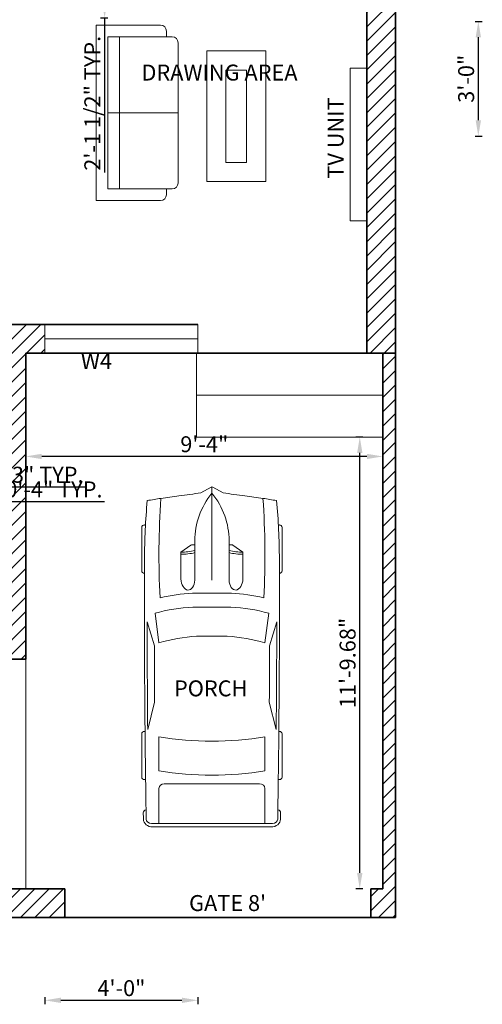
# Model space of a CAD drawing. Units: inches. Extents: x -196 to 219, y -474 to 80.
# Tile 3 of 4: x 73 to 219, y -456 to -148. Entities that reach past the tile are written whole.
import ezdxf

# ---------------------------------------------------------------- set-up
doc = ezdxf.new("R2010")
doc.units = ezdxf.units.IN
doc.header["$PDMODE"] = 35
doc.header["$PDSIZE"] = 5
for name, color, linetype, lineweight in [('A-ANNO-DIMS', 2, 'Continuous', 18), ('A-ANNO-TEXT', 7, 'Continuous', 18), ('A-AREA-IDEN', 7, 'Continuous', 25), ('A-FLOR-STRS', 3, 'Continuous', 18), ('A-GLAZ', 4, 'Continuous', 18), ('A-SITE-VEHI', 8, 'Continuous', 13), ('A-WALL', 7, 'Continuous', 35), ('A-WALL-PATT', 252, 'Continuous', 13), ('A-WALL-SITE', 7, 'Continuous', 35), ('furn', 28, 'Continuous', 18)]:
    doc.layers.add(name, color=color, linetype=linetype, lineweight=lineweight)
doc.styles.get("Standard").update_dxf_attribs({"font": 'arial.ttf'})
doc.dimstyles.new('ISO-25', dxfattribs={"dimtxt": 5, "dimasz": 5, "dimexe": 1.25, "dimexo": 0.625, "dimtad": 1, "dimlunit": 3, "dimtxsty": 'Standard', "dimcen": 2.5, "dimadec": 0, "dimazin": 0, "dimtfac": 1, "dimtmove": 0, "dimatfit": 3, "dimfxl": 1, "dimfxlon": 1, "dimarcsym": 0})

# ---------------------------------------------------------------- blocks, each defined once
blk = doc.blocks.new('sofa-6')
at = {"color": 0, "linetype": 'ByBlock'}
for p, q in [((1.35, 0.7), (0.15, 0.7)), ((0.75, 0.1), (0.75, 0.7)), ((0.1, 0.6), (0.05, 0.6)), ((0.1, 0.65), (0.1, 0.1)), ((1.4, 0.1), (1.4, 0.65)), ((1.45, 0.6), (1.4, 0.6)), ((0, 0.55), (0, 0)), ((1.5, 0), (1.5, 0.55)), ((0.1, 0.2), (1.4, 0.2)), ((0.1, 0.1), (1.4, 0.1)), ((0, 0), (1.5, 0))]:
    blk.add_line(p, q, dxfattribs=at)
for centre, start, end in [((0.15, 0.65), 90, 180), ((1.35, 0.65), 360, 90), ((0.05, 0.55), 90, 180), ((1.45, 0.55), 0, 90)]:
    blk.add_arc(centre, 0.05, start, end, dxfattribs=at)
blk = doc.blocks.new('*U24')
for p, q in [((46.55, 38.89), (22.35, 38.89)), ((136.7, 38.89), (160.9, 38.89)), ((21.1, 37.41), (21.1, 36.83)), ((47.8, 37.39), (47.8, 37.41)), ((87.99, 31.87), (74.76, 35.92)), ((134.31, 35.6), (119.29, 31.78)), ((135.45, 37.07), (135.45, 37.41)), ((162.15, 37.41), (162.15, 36.77)), ((186.47, -33.5), (186.47, 33.5)), ((188.4, -32.76), (188.4, 32.76)), ((70.03, 31.54), (86.41, 29.35)), ((138.42, 29.35), (157.25, 29.35)), ((186.47, 29.35), (167.01, 29.35)), ((164.52, 26.39), (164.52, -26.39)), ((32.27, 11.63), (36.13, 17.17)), ((36.13, 17.17), (50.94, 17.17)), ((32.12, 9.51), (32.12, 11.15)), ((3.27, 6.13), (0.1, 0.41)), ((29.77, 9.51), (51.68, 9.51)), ((58.92, -10.77), (58.92, 10.77)), ((66.55, -10.53), (66.55, 10.53)), ((82.74, 8.5), (82.74, -8.5)), ((186.47, -10.53), (186.47, 10.53)), ((0, 0), (51.68, 0)), ((0.1, -0.41), (3.27, -6.13)), ((29.77, -9.51), (51.68, -9.51)), ((32.12, -9.51), (32.12, -11.15)), ((32.27, -11.63), (36.13, -17.17)), ((36.13, -17.17), (50.94, -17.17)), ((86.41, -29.35), (70.03, -31.54)), ((87.99, -31.87), (74.76, -35.92)), ((134.31, -35.6), (119.29, -31.78)), ((157.25, -29.35), (138.42, -29.35)), ((167.01, -29.35), (186.47, -29.35)), ((21.1, -37.41), (21.1, -36.83)), ((47.8, -37.39), (47.8, -37.41)), ((135.45, -37.07), (135.45, -37.41)), ((162.15, -37.41), (162.15, -36.77)), ((46.55, -38.89), (22.35, -38.89)), ((136.7, -38.89), (160.9, -38.89))]:
    blk.add_line(p, q)
for centre, major_axis, ratio, start_param, end_param in [((22.35, 37.41), (0, -1.48), 0.842304, 3.141593, 4.712389), ((46.55, 37.41), (0, 1.48), 0.842304, -1.570796, 0), ((136.7, 37.41), (0, -1.48), 0.842304, 3.141593, 4.712389), ((160.9, 37.41), (0, 1.48), 0.842304, -1.570796, 0), ((266.03, -27.52), (0, 313.31), 0.842304, 1.367076, 1.39176), ((41.19, -490.86), (0, 528.23), 0.842304, 0.00281, 0.075598), ((64.48, -10555.62), (0, 10593.03), 0.842304, -0.013397, 0.002797), ((64.48, -10555.62), (0, -10591.55), 0.842304, 3.133765, 3.140441), ((180.63, 35.84), (0, 2.22), 0.842304, -0.013017, 1.249894), ((64.48, -10556.36), (0, 10595.31), 0.842304, -0.013397, -0.013017), ((183.98, 33.5), (0, -2.96), 0.842304, 1.570796, 3.128196), ((183.98, 32.76), (0, -5.25), 0.842304, 1.570796, 3.128196), ((259.18, -27.52), (0, -305.3), 0.842304, 4.528606, 4.561838), ((37.47, -593.96), (0, -623.33), 0.842304, 3.096046, 3.200911), ((134.4, 5.39), (0, -89.78), 0.842304, 4.449482, 4.652344), ((135.29, 5.39), (0, 81.77), 0.842304, 1.245306, 1.50788), ((149.6, 2.8), (0, -79.58), 0.842304, 4.372215, 4.640744), ((95.79, -3666.35), (0, -3698.24), 0.842304, 3.134049, 3.144098), ((17.08, 0), (0, 147.02), 0.842304, 4.511394, 4.913384), ((35.91, 0), (0, 147.02), 0.842304, 4.511394, 4.913384), ((167.01, 26.39), (0, 2.96), 0.842304, 0, 1.570796), ((-204.49, 52.4), (0, -250.96), 0.842304, 1.385369, 1.434372), ((13.04, 17.01), (0, 27.42), 0.842304, 4.435146, 4.718221), ((14.2, 17.01), (0, 27.42), 0.842304, 4.435146, 4.718221), ((50.79, 13.34), (6.34, -0.36), 0.603834, -1.395552, 1.581315), ((32.75, 11.15), (0, 0.74), 0.842304, 0.879714, 1.570796), ((29.77, -46.66), (0, 56.17), 0.842304, 0, 0.590319), ((0.62, 0), (0, -0.74), 0.842304, 4.131459, 5.293319), ((29.77, 46.66), (0, 56.17), 0.842304, 2.551274, 3.141593), ((-204.49, -52.4), (0, 250.96), 0.842304, -1.434372, -1.385369), ((13.04, -17.01), (0, -27.42), 0.842304, 1.564964, 1.848039), ((14.2, -17.01), (0, -27.42), 0.842304, 1.564964, 1.848039), ((134.4, -5.39), (0, -89.78), 0.842304, -1.510751, -1.307889), ((135.29, -5.39), (0, -81.77), 0.842304, -1.50788, -1.245306), ((149.6, -2.8), (0, -79.58), 0.842304, -1.499151, -1.230623), ((32.75, -11.15), (0, -0.74), 0.842304, 4.712389, 5.403472), ((259.18, 27.52), (0, 305.3), 0.842304, 1.721348, 1.754579), ((167.01, -26.39), (0, -2.96), 0.842304, 4.712389, 6.283185), ((266.03, 27.52), (0, 313.31), 0.842304, 1.749832, 1.774517), ((37.47, 593.96), (0, -623.33), 0.842304, -0.059319, 0.045547), ((95.79, 3666.35), (0, -3698.24), 0.842304, -0.002505, 0.007544), ((41.19, 490.86), (0, -528.23), 0.842304, -0.075598, -0.00281), ((22.35, -37.41), (0, 1.48), 0.842304, 1.570796, 3.141593), ((64.48, 10555.62), (0, 10593.03), 0.842304, 3.138796, 3.15499), ((46.55, -37.41), (0, -1.48), 0.842304, 0, 1.570796), ((64.48, 10555.62), (0, -10591.55), 0.842304, 0.001152, 0.007828), ((136.7, -37.41), (0, -1.48), 0.842304, -1.570796, 0), ((160.9, -37.41), (0, 1.48), 0.842304, 3.141593, 4.712389), ((180.63, -35.84), (0, -2.22), 0.842304, -1.249894, 0.013017), ((64.48, 10556.36), (0, 10595.31), 0.842304, 3.15461, 3.15499), ((183.98, -33.5), (0, 2.96), 0.842304, 3.15499, 4.712389), ((183.98, -32.76), (0, -5.25), 0.842304, 0.013397, 1.570796)]:
    blk.add_ellipse(centre, major_axis=major_axis, ratio=ratio, start_param=start_param, end_param=end_param)
at = {"extrusion": (0, 0, -1)}
blk.add_ellipse((50.79, -13.34), major_axis=(6.34, 0.36), ratio=0.603834, start_param=-1.395552, end_param=1.581315, dxfattribs=at)
blk = doc.blocks.new('*D27')
at = {"layer": 'A-ANNO-DIMS', "color": 0, "lineweight": -2, "transparency": 16777216}
for p, q in [((181.06, -278.42), (178.81, -278.42)), ((180.06, -415.09), (180.06, -283.42)), ((181.06, -420.09), (178.81, -420.09))]:
    blk.add_line(p, q, dxfattribs=at)
at = {"layer": 'A-ANNO-DIMS', "color": 0, "transparency": 16777216}
for points in [[(179.23, -283.42), (180.9, -283.42), (180.06, -278.42)], [(179.23, -415.09), (180.9, -415.09), (180.06, -420.09)]]:
    blk.add_solid(points, dxfattribs=at)
at = {"layer": 'Defpoints', "color": 0, "transparency": 16777216}
for p in [(180.06, -278.42), (187.3, -278.42), (187.3, -420.09)]:
    blk.add_point(p, dxfattribs=at)
at = {"layer": 'A-ANNO-DIMS', "color": 0, "transparency": 16777216, "insert": (176.89, -349.26), "char_height": 5, "attachment_point": 5, "rotation": 90}
blk.add_mtext('11\'-9.68"', dxfattribs=at)
blk = doc.blocks.new('*D28')
at = {"layer": 'A-ANNO-DIMS', "color": 0, "lineweight": -2, "transparency": 16777216}
for p, q in [((75.3, -284.51), (75.3, -283.26)), ((187.3, -283.51), (187.3, -285.76)), ((182.3, -284.51), (80.3, -284.51))]:
    blk.add_line(p, q, dxfattribs=at)
at = {"layer": 'A-ANNO-DIMS', "color": 0, "transparency": 16777216}
for points in [[(80.3, -283.68), (80.3, -285.34), (75.3, -284.51)], [(182.3, -283.68), (182.3, -285.34), (187.3, -284.51)]]:
    blk.add_solid(points, dxfattribs=at)
at = {"layer": 'Defpoints', "color": 0, "transparency": 16777216}
for p in [(187.3, -278.42), (75.3, -284.51), (75.3, -284.51)]:
    blk.add_point(p, dxfattribs=at)
at = {"layer": 'A-ANNO-DIMS', "color": 0, "transparency": 16777216, "insert": (131.3, -281.33), "char_height": 5, "attachment_point": 5}
blk.add_mtext('9\'-4"', dxfattribs=at)
blk = doc.blocks.new('*D45')
at = {"layer": 'A-ANNO-DIMS', "color": 0, "lineweight": -2, "transparency": 16777216}
for p, q in [((101.03, -121.37), (98.78, -121.37)), ((100.03, -126.37), (100.03, -142.04)), ((101.03, -147.04), (98.78, -147.04)), ((100.03, -147.04), (100.03, -195.5))]:
    blk.add_line(p, q, dxfattribs=at)
at = {"layer": 'A-ANNO-DIMS', "color": 0, "transparency": 16777216}
for points in [[(99.19, -126.37), (100.86, -126.37), (100.03, -121.37)], [(99.19, -142.04), (100.86, -142.04), (100.03, -147.04)]]:
    blk.add_solid(points, dxfattribs=at)
at = {"layer": 'Defpoints', "color": 0, "transparency": 16777216}
for p in [(108.28, -121.37), (100.03, -147.04), (108.28, -147.04)]:
    blk.add_point(p, dxfattribs=at)
at = {"layer": 'A-ANNO-DIMS', "color": 0, "transparency": 16777216, "insert": (96.82, -173.77), "char_height": 5, "attachment_point": 5, "rotation": 90}
blk.add_mtext('2\'-1 1/2" TYP.', dxfattribs=at)
blk = doc.blocks.new('*D49')
at = {"layer": 'A-ANNO-DIMS', "color": 0, "lineweight": -2, "transparency": 16777216}
for p, q in [((49.1, -298.67), (44.1, -298.67)), ((54.1, -298.67), (54.1, -299.92)), ((54.1, -298.67), (58.25, -298.67)), ((58.25, -298.67), (58.25, -299.92)), ((63.25, -298.67), (99.98, -298.67))]:
    blk.add_line(p, q, dxfattribs=at)
at = {"layer": 'A-ANNO-DIMS', "color": 0, "transparency": 16777216}
for points in [[(49.1, -297.83), (49.1, -299.5), (54.1, -298.67)], [(63.25, -297.83), (63.25, -299.5), (58.25, -298.67)]]:
    blk.add_solid(points, dxfattribs=at)
at = {"layer": 'Defpoints', "color": 0, "transparency": 16777216}
for p in [(54.1, -298.04), (58.25, -298.04), (58.25, -298.67)]:
    blk.add_point(p, dxfattribs=at)
at = {"layer": 'A-ANNO-DIMS', "color": 0, "transparency": 16777216, "insert": (84.11, -295.49), "char_height": 5, "attachment_point": 5}
blk.add_mtext('0\'-4" TYP.', dxfattribs=at)
blk = doc.blocks.new('*D51')
at = {"layer": 'A-ANNO-DIMS', "color": 0, "lineweight": -2, "transparency": 16777216}
for p, q in [((49.39, -294.07), (49.39, -292.82)), ((52.3, -294.07), (52.3, -292.82)), ((44.39, -294.07), (39.39, -294.07)), ((49.39, -294.07), (52.3, -294.07)), ((57.3, -294.07), (94.02, -294.07))]:
    blk.add_line(p, q, dxfattribs=at)
at = {"layer": 'A-ANNO-DIMS', "color": 0, "transparency": 16777216}
for points in [[(44.39, -293.23), (44.39, -294.9), (49.39, -294.07)], [(57.3, -293.23), (57.3, -294.9), (52.3, -294.07)]]:
    blk.add_solid(points, dxfattribs=at)
at = {"layer": 'Defpoints', "color": 0, "transparency": 16777216}
for p in [(49.39, -294.5), (52.3, -294.07), (52.3, -294.5)]:
    blk.add_point(p, dxfattribs=at)
at = {"layer": 'A-ANNO-DIMS', "color": 0, "transparency": 16777216, "insert": (78.16, -290.89), "char_height": 5, "attachment_point": 5}
blk.add_mtext('0\'-3" TYP.', dxfattribs=at)
blk = doc.blocks.new('*D56')
at = {"layer": 'A-ANNO-DIMS', "color": 0, "lineweight": -2, "transparency": 16777216}
for p, q in [((216.25, -148.09), (218.5, -148.09)), ((217.25, -153.09), (217.25, -179.09)), ((216.25, -184.09), (218.5, -184.09))]:
    blk.add_line(p, q, dxfattribs=at)
at = {"layer": 'A-ANNO-DIMS', "color": 0, "transparency": 16777216}
for points in [[(216.42, -153.09), (218.09, -153.09), (217.25, -148.09)], [(216.42, -179.09), (218.09, -179.09), (217.25, -184.09)]]:
    blk.add_solid(points, dxfattribs=at)
at = {"layer": 'Defpoints', "color": 0, "transparency": 16777216}
for p in [(-35.7, -148.09), (-35.7, -184.09), (217.25, -184.09)]:
    blk.add_point(p, dxfattribs=at)
at = {"layer": 'A-ANNO-DIMS', "color": 0, "transparency": 16777216, "insert": (214.07, -166.09), "char_height": 5, "attachment_point": 5, "rotation": 90}
blk.add_mtext('3\'-0"', dxfattribs=at)
blk = doc.blocks.new('*D59')
at = {"layer": 'A-ANNO-DIMS', "color": 0, "lineweight": -2, "transparency": 16777216}
for p, q in [((81.3, -454.04), (81.3, -456.29)), ((86.3, -455.04), (124.3, -455.04)), ((129.3, -454.04), (129.3, -456.29))]:
    blk.add_line(p, q, dxfattribs=at)
at = {"layer": 'A-ANNO-DIMS', "color": 0, "transparency": 16777216}
for points in [[(86.3, -454.21), (86.3, -455.88), (81.3, -455.04)], [(124.3, -454.21), (124.3, -455.88), (129.3, -455.04)]]:
    blk.add_solid(points, dxfattribs=at)
at = {"layer": 'Defpoints', "color": 0, "transparency": 16777216}
for p in [(81.3, -252.09), (129.3, -252.09), (129.3, -455.04)]:
    blk.add_point(p, dxfattribs=at)
at = {"layer": 'A-ANNO-DIMS', "color": 0, "transparency": 16777216, "insert": (105.3, -451.87), "char_height": 5, "attachment_point": 5}
blk.add_mtext('4\'-0"', dxfattribs=at)
blk = doc.blocks.new('*D60')
at = {"layer": 'A-ANNO-DIMS', "color": 0, "lineweight": -2, "transparency": 16777216}
for p, q in [((66.3, 72.61), (66.3, 74.86)), ((75.3, 72.61), (75.3, 74.86)), ((61.3, 73.61), (56.3, 73.61)), ((66.3, 73.61), (75.3, 73.61)), ((80.3, 73.61), (99.84, 73.61))]:
    blk.add_line(p, q, dxfattribs=at)
at = {"layer": 'A-ANNO-DIMS', "color": 0, "transparency": 16777216}
for points in [[(61.3, 74.45), (61.3, 72.78), (66.3, 73.61)], [(80.3, 74.45), (80.3, 72.78), (75.3, 73.61)]]:
    blk.add_solid(points, dxfattribs=at)
at = {"layer": 'Defpoints', "color": 0, "transparency": 16777216}
for p in [(75.3, 73.61), (66.3, -339.09), (75.3, -348.09)]:
    blk.add_point(p, dxfattribs=at)
at = {"layer": 'A-ANNO-DIMS', "color": 0, "transparency": 16777216, "insert": (92.57, 76.79), "char_height": 5, "attachment_point": 5}
blk.add_mtext('0\'-9"', dxfattribs=at)

msp = doc.modelspace()

# ---------------------------------------------------------------- hatches: boundary and pattern name
at = {"layer": 'A-WALL-PATT'}
h = msp.add_hatch(dxfattribs=at)
h.set_pattern_fill('ANSI31', color=256)
h.set_pattern_definition([(45, (-560.5042, 72.7454), (-2.245064, 2.245064), [])])
h.paths.add_polyline_path([(-159.698, -243.094), (-159.698, -148.094), (-159.698, 23.906), (-39.698, 23.906), (-39.698, -108.969), (-35.698, -108.969), (-35.698, -105.094), (-23.894, -105.094), (-23.894, -96.094), (-35.698, -96.094), (-35.698, -64.094), (-21.698, -64.094), (-21.698, -60.094), (-35.698, -60.094), (-35.698, -12.094), (-24.951, -12.094), (-24.951, -8.094), (-35.698, -8.094), (-35.698, 23.906), (-35.698, 27.906), (60.302, 27.906), (60.302, 23.906), (60.302, -8.094), (42.302, -8.094), (42.302, -12.094), (60.302, -12.094), (60.302, -96.094), (42.302, -96.094), (8.302, -96.094), (8.302, -105.094), (42.302, -105.094), (60.302, -105.094), (64.302, -105.094), (64.302, 23.906), (182.302, 23.906), (182.302, -96.094), (100.302, -96.094), (100.302, -105.094), (182.302, -105.094), (182.302, -252.094), (191.302, -252.094), (191.302, 32.906), (-168.698, 32.906), (-168.698, -399.094), (-134.786, -399.094), (-134.786, -390.094), (-159.698, -390.094)])
h.paths.add_polyline_path([(191.302, -252.094), (187.302, -252.094), (187.302, -420.094), (183.555, -420.094), (183.555, -429.094), (191.302, -429.094)])
h.paths.add_polyline_path([(87.555, -420.094), (75.302, -420.094), (38.543, -420.094), (3.06, -420.094), (3.06, -425.094), (3.06, -429.094), (87.555, -429.094)])
h.paths.add_polyline_path([(75.302, -252.094), (81.302, -252.094), (81.302, -243.094), (0.302, -243.094), (0.302, -252.094), (66.302, -252.094), (66.302, -339.094), (37.784, -339.094), (37.784, -348.094), (66.302, -348.094), (75.302, -348.094)], flags=17)
h.paths.add_polyline_path([(-16.216, -339.094), (-35.698, -339.094), (-35.698, -243.094), (-43.698, -243.094), (-43.698, -252.094), (-39.698, -252.094), (-39.698, -352.094), (-35.698, -352.094), (-35.698, -348.094), (-16.216, -348.094)], flags=17)
h.paths.add_polyline_path([(-79.698, -243.094), (-159.698, -243.094), (-159.698, -252.094), (-79.698, -252.094)], flags=17)
h.paths.add_polyline_path([(-35.698, -144.094), (-159.698, -144.094), (-159.698, -148.094), (-35.698, -148.094)], flags=17)

# ---------------------------------------------------------------- linework, layer by layer
at = {"layer": 'A-FLOR-STRS'}
for p, q in [((128.802, -252.094), (128.802, -278.417)), ((128.802, -265.255), (187.302, -265.255)), ((128.802, -278.417), (187.302, -278.417)), ((75.302, -348.094), (75.302, -420.094))]:
    msp.add_line(p, q, dxfattribs=at)
at = {"layer": 'A-GLAZ'}
for p, q in [((81.302, -252.094), (81.302, -243.094)), ((129.302, -252.094), (129.302, -243.094)), ((81.302, -247.594), (129.302, -247.594))]:
    msp.add_line(p, q, dxfattribs=at)
at = {"layer": 'A-WALL'}
for p, q in [((191.302, 32.906), (191.302, -252.094)), ((182.302, -105.094), (182.302, -252.094)), ((129.302, -243.094), (-159.698, -243.094)), ((182.302, -252.094), (75.302, -252.094)), ((75.302, -252.094), (75.302, -348.094)), ((182.302, -252.094), (191.302, -252.094)), ((66.302, -348.094), (75.302, -348.094))]:
    msp.add_line(p, q, dxfattribs=at)
at = {"layer": 'A-WALL-SITE'}
for p, q in [((187.302, -252.094), (187.302, -420.094)), ((191.302, -252.094), (191.302, -429.094)), ((38.543, -420.094), (75.302, -420.094)), ((75.302, -420.094), (87.555, -420.094)), ((87.555, -420.094), (87.555, -429.094)), ((183.555, -420.094), (183.555, -429.094)), ((183.555, -420.094), (187.302, -420.094)), ((3.06, -429.094), (191.302, -429.094))]:
    msp.add_line(p, q, dxfattribs=at)
at = {"layer": 'furn'}
for points in [[(132.063, -157.381), (150.552, -157.381), (150.552, -198.311), (132.063, -198.311)], [(138.063, -163.381), (144.552, -163.381), (144.552, -192.311), (138.063, -192.311)], [(182.302, -162.722), (177.015, -162.722), (177.015, -210.63), (182.302, -210.63)]]:
    msp.add_lwpolyline(points, close=True, dxfattribs=at)

# ---------------------------------------------------------------- block references
at = {"layer": 'A-SITE-VEHI', "xscale": 0.5659501802745862, "yscale": 0.5659501802745862, "zscale": 0.5659501802745862, "rotation": 270}
msp.add_blockref('*U24', (133.694, -294.064), dxfattribs=at)
at = {"layer": 'furn', "xscale": 36.66436083614781, "yscale": 36.66436083614781, "zscale": 36.66436083614781, "rotation": 270}
msp.add_blockref('sofa-6', (97.403, -149.279), dxfattribs=at)

# ---------------------------------------------------------------- texts
at = {"layer": 'A-ANNO-TEXT', "insert": (170.017, -197.406), "char_height": 5, "attachment_point": 1, "rotation": 90}
msp.add_mtext_dynamic_manual_height_columns('TV UNIT', width=63.32292, gutter_width=12.5, heights=[0], dxfattribs=at)
at = {"layer": 'A-ANNO-TEXT', "char_height": 5, "attachment_point": 1}
for s, width, insert in [('W4', 26.04527, (92.567, -252.094)), ("GATE 8'", 37.18399, (126.525, -422.048))]:
    msp.add_mtext_dynamic_manual_height_columns(s, width=width, gutter_width=12.5, heights=[0], dxfattribs=dict(at, insert=insert))
at = {"layer": 'A-AREA-IDEN', "char_height": 5, "attachment_point": 1}
for s, width, insert in [('DRAWING AREA', 68.26999, (111.582, -161.645)), ('PORCH', 39.97524, (121.791, -354.73))]:
    msp.add_mtext_dynamic_manual_height_columns(s, width=width, gutter_width=12.5, heights=[0], dxfattribs=dict(at, insert=insert))

# ---------------------------------------------------------------- dimensions: what is measured, and where the dimension line sits
at = {"layer": 'A-ANNO-DIMS'}
for base, p1, p2, override, picture, middle in [((75.302, 73.612), (66.302, -339.094), (75.302, -348.094), {"dimdec": 1, "dimlfac": 1, "dimrnd": 0, "dimzin": 1, "dimdsep": 46, "dimlunit": 4, "dimfrac": 2}, '*D60', (92.573, 76.79)), ((129.302, -455.044), (81.302, -252.094), (129.302, -252.094), {"dimdec": 1, "dimlfac": 1, "dimrnd": 0, "dimzin": 1, "dimdsep": 46, "dimlunit": 4, "dimfrac": 2}, '*D59', (105.302, -451.866)), ((75.302, -284.51), (187.302, -278.417), (75.302, -284.51), {"dimclrd": 0, "dimclre": 0, "dimclrt": 0}, '*D28', (131.302, -281.332))]:
    dim = msp.add_linear_dim(base=base, p1=p1, p2=p2, dimstyle='ISO-25', override=override, dxfattribs=at)
    dim.commit()
    dim.dimension.update_dxf_attribs({"geometry": picture, "text_midpoint": middle})
dim = msp.add_linear_dim(base=(100.027, -147.037), p1=(108.276, -121.371), p2=(108.276, -147.037), angle=270, text='<> TYP.', dimstyle='ISO-25', override={"dimdec": 1, "dimlfac": 1, "dimrnd": 0, "dimzin": 1, "dimdsep": 46, "dimlunit": 4, "dimfrac": 2}, dxfattribs=at)
dim.commit()
dim.dimension.update_dxf_attribs({"geometry": '*D45', "text_midpoint": (96.817, -173.768)})
for base, p1, p2, override, picture, middle in [((217.252, -184.094), (-35.698, -148.094), (-35.698, -184.094), {"dimdec": 1, "dimlfac": 1, "dimrnd": 0, "dimzin": 1, "dimdsep": 46, "dimlunit": 4, "dimfrac": 2}, '*D56', (214.072, -166.094)), ((180.064, -278.417), (187.302, -420.094), (187.302, -278.417), {"dimclrd": 0, "dimclre": 0, "dimclrt": 0}, '*D27', (176.886, -349.255))]:
    dim = msp.add_linear_dim(base=base, p1=p1, p2=p2, angle=90, dimstyle='ISO-25', override=override, dxfattribs=at)
    dim.commit()
    dim.dimension.update_dxf_attribs({"geometry": picture, "text_midpoint": middle})
for base, p1, p2, picture, middle in [((52.297, -294.066), (49.389, -294.505), (52.297, -294.505), '*D51', (78.161, -290.886)), ((58.25, -298.667), (54.096, -298.041), (58.25, -298.041), '*D49', (84.114, -295.489))]:
    dim = msp.add_linear_dim(base=base, p1=p1, p2=p2, text='<> TYP.', dimstyle='ISO-25', override={"dimdec": 1, "dimlfac": 1, "dimrnd": 0, "dimzin": 1, "dimdsep": 46, "dimlunit": 4, "dimfrac": 2}, dxfattribs=at)
    dim.commit()
    dim.dimension.update_dxf_attribs({"geometry": picture, "text_midpoint": middle})

doc.saveas('drawing.dxf')
